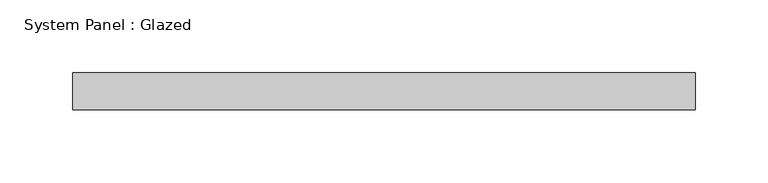
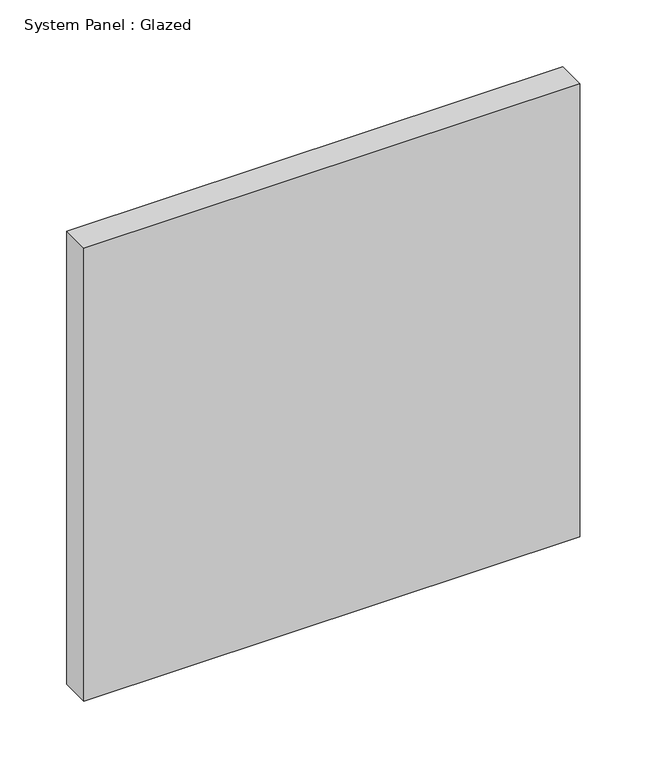
"""IFC4 building model written with IfcOpenShell, lengths in millimetres: plate geometry, System Panel : Glazed."""

from ifc_helpers import new_model, si_unit, origin, origin_with_axes, place, context, project, spatial, polyline, outline, extrude, source, transform, mapped, element, save


def system_panel_glazed_c56bea94(model_context):
    return source(origin(), model_context, "Body", "SweptSolid", [
        extrude(outline(polyline([(213.7833333, 19.05), (-213.7833333, 19.05), (-213.7833333, 44.45), (213.7833333, 44.45), (213.7833333, 19.05)])), origin_with_axes(), (0.0, 0.0, 1.0), 412.75),
    ])


if __name__ == "__main__":
    model = new_model("IFC4")
    model_context = context("Model", 3, world=origin())
    ifc_project = project(units=[si_unit("LENGTHUNIT", "METRE", prefix="MILLI")], contexts=[model_context])
    site = spatial("IfcSite", under=ifc_project)
    building = spatial("IfcBuilding", under=site)
    placement = place(None, origin())
    system_panel_glazed_shape = system_panel_glazed_c56bea94(model_context)
    element("IfcPlate", 1, ObjectType="System Panel : Glazed", at=placement, inside=building, context=model_context, shape_type="MappedRepresentation", body=[
        mapped(system_panel_glazed_shape, transform((0.0, 0.0, 0.0), x_axis=(1.0, 0.0, 0.0), y_axis=(0.0, 1.0, 0.0), z_axis=(0.0, 0.0, 1.0))),
    ])
    save(model, "model.ifc")

# Revit data of these elements
# Type "System Panel : Glazed"
#   Construction Type Id = "GSP4R"
#   Analytic Construction = "1/8 in Pilkington single glazing"
#   Visual Light Transmittance = 0.9
#   Solar Heat Gain Coefficient = 0.86
#   Heat Transfer Coefficient (U) = 1.18115 BTU/(h·ft²·°F)
#   Define Thermal Properties by = 1
# Element 1 (IfcPlate, "System Panel : Glazed")
#   Materials on its faces: "Glass"
# Materials
#   "Glass": class "Glass", colour RGB 0 128 192, transparency 0.75, Description = "Soda Lime Glass", Cost = 0
